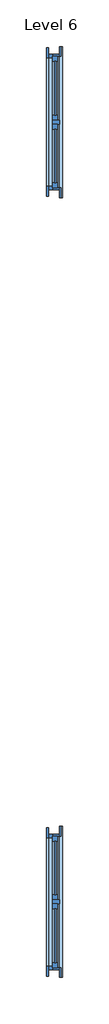
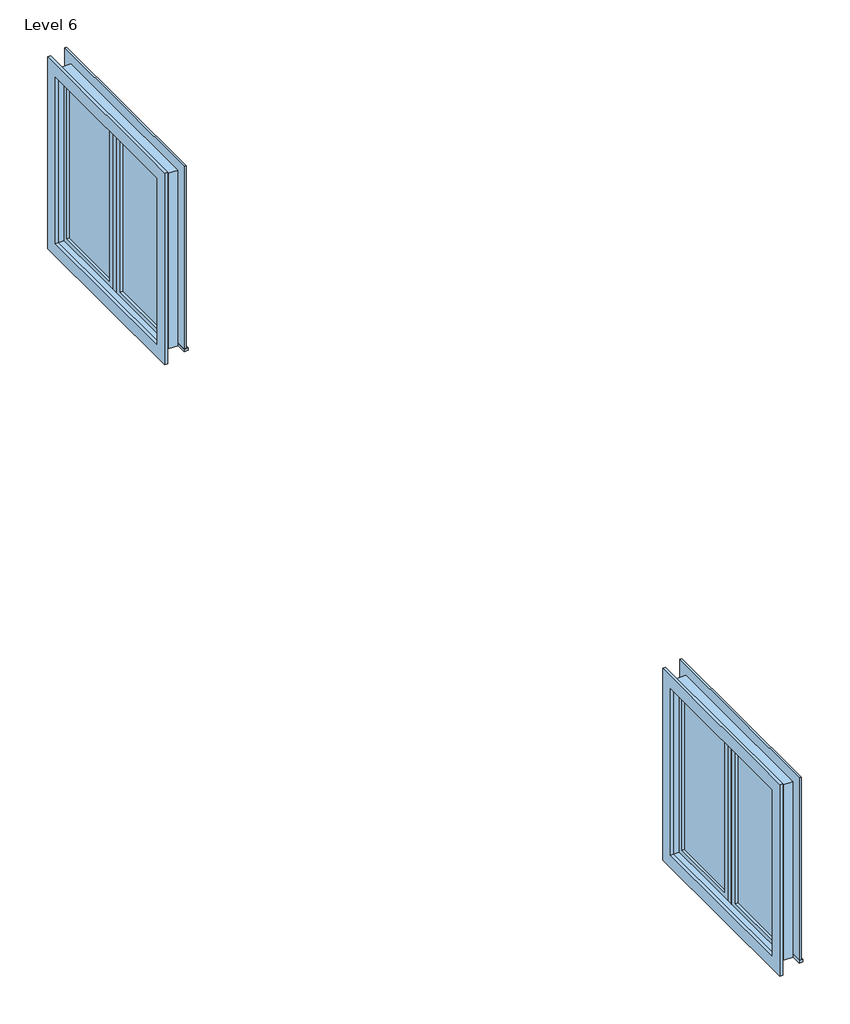
# One storey: 2 windows.
"""IFC4 building model written with IfcOpenShell, lengths in millimetres."""

from ifc_helpers import new_model, si_unit, origin, place, context, project, spatial, transform, mapped, element, save
from components import window_90ef9153

model = new_model("IFC4")

# Units and contexts
model_context = context("Model", 3, world=origin())
ifc_project = project(units=[si_unit("LENGTHUNIT", "METRE", prefix="MILLI")], contexts=[model_context])

# Site, building, storey
site = spatial("IfcSite", under=ifc_project)
building = spatial("IfcBuilding", under=site)
storey = spatial("IfcBuildingStorey", under=building, Name="Level 6", Elevation=9448.8)

# Windows
placement = place(None, origin())
window_shape = window_90ef9153(model_context)
element("IfcWindow", 1, ObjectType="Casement Dbl with Trim : 48\" x 48\"", at=placement, inside=storey, context=model_context, shape_type="MappedRepresentation", body=[
    mapped(window_shape, transform((13917.4668112, 1971.5281796, 9448.8), x_axis=(0.0, -1.0, 0.0), y_axis=(1.0, 0.0, 0.0), z_axis=(0.0, 0.0, 1.0))),
])
element("IfcWindow", 2, ObjectType="Casement Dbl with Trim : 48\" x 48\"", at=placement, inside=storey, context=model_context, shape_type="MappedRepresentation", body=[
    mapped(window_shape, transform((13917.4668112, 8981.9281796, 9448.8), x_axis=(0.0, -1.0, 0.0), y_axis=(1.0, 0.0, 0.0), z_axis=(0.0, 0.0, 1.0))),
])

save(model, "model.ifc")

# Revit data of these elements
# Type "Casement Dbl with Trim : 48\" x 48\""
#   Type Mark = "13"
#   Construction Type Id = "GSP4R"
#   Assembly Code = "B2020100"
#   Analytic Construction = "1/8 in Pilkington single glazing"
#   Visual Light Transmittance = 0.9
#   Solar Heat Gain Coefficient = 0.78
#   Heat Transfer Coefficient (U) = 0.6496 BTU/(h·ft²·°F)
#   Height = 4' - 0"
#   Default Sill Height = 3' - 0"
#   Trim Projection - Ext. = 0' - 0 1/2"
#   Trim Projection - Int. = 0' - 0 3/4"
#   Trim Width - Exterior = 0' - 3 1/2"
#   Trim Width - Interior = 0' - 3 1/2"
#   Width = 4' - 0"
#   Window Inset = 0' - 0 3/4"
#   Define Thermal Properties by = 1
#   Glass Pane Material = Glass
#   Sash Material = Sash
#   Trim Exterior Material = Trim
#   Trim Interior Material = Trim
#   Wall Closure = (empty or 0)
# Element 1 (IfcWindow, "Casement Dbl with Trim : 48\" x 48\"")
#   Mark = "23"
#   Phase Created = New Construction
#   Materials on its faces: "Sash", "Trim", "Glass"
# Element 2 (IfcWindow, "Casement Dbl with Trim : 48\" x 48\"")
#   Mark = "24"
#   Phase Created = New Construction
#   Materials on its faces: "Sash", "Trim", "Glass"
# Materials
#   "Glass": class "Glass", colour RGB 0 128 192, transparency 0.75, Description = "Soda Lime Glass", Cost = 0
#   "Sash": class "Wood", colour RGB 224 178 126, transparency 0
#   "Trim": class "Wood", colour RGB 224 178 126, transparency 0
